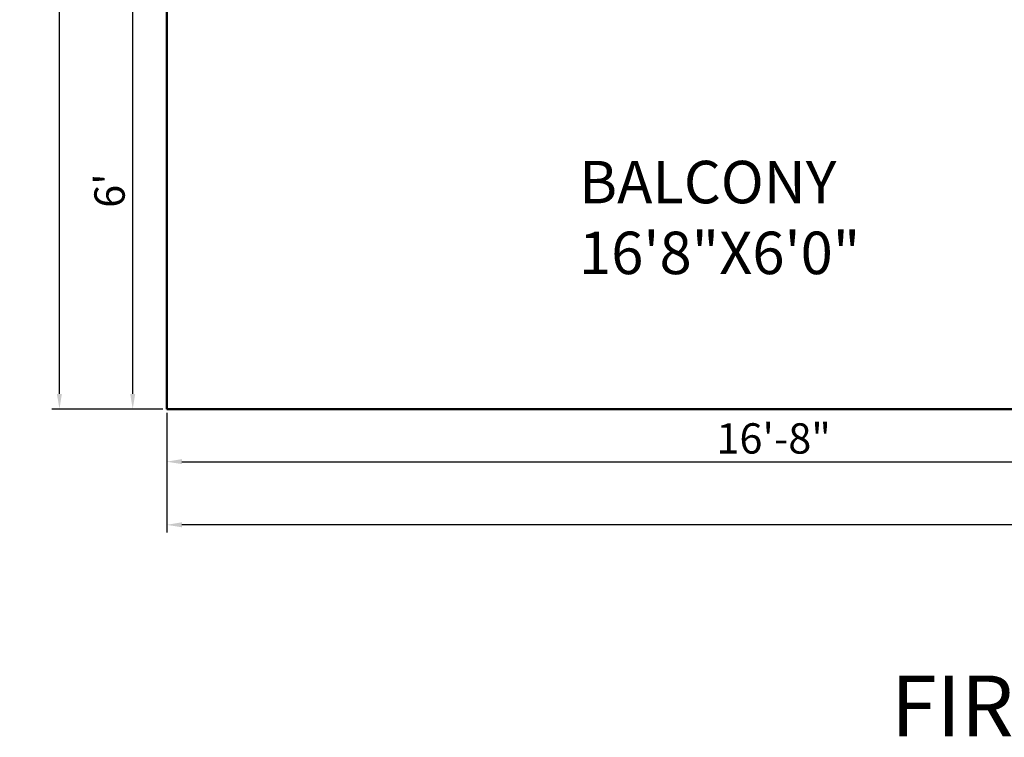
# Model space of a CAD drawing. Units: inches. Extents: x 3064 to 19385, y 846 to 15425.
# Tile 35 of 108: x 5167 to 5329, y 846 to 964. Entities that reach past the tile are written whole.
import ezdxf

# ---------------------------------------------------------------- set-up
doc = ezdxf.new("R2010")
doc.units = ezdxf.units.IN
for name, color, linetype, lineweight in [('A-ANNO-DIMS', 2, 'Continuous', 18), ('A-ANNO-TEXT', 7, 'Continuous', 25), ('A-AREA-IDEN', 3, 'Continuous', 18), ('A-WALL', 7, 'Continuous', 50)]:
    doc.layers.add(name, color=color, linetype=linetype, lineweight=lineweight)
doc.styles.get("Standard").update_dxf_attribs({"font": 'arial.ttf'})
doc.dimstyles.new('ISO-25', dxfattribs={"dimtxt": 9, "dimasz": 2.5, "dimexe": 1.25, "dimexo": 0.625, "dimtad": 1, "dimdec": 1, "dimlunit": 3, "dimtxsty": 'Standard', "dimcen": 2.5, "dimadec": 0, "dimazin": 0, "dimtfac": 1, "dimtdec": 1, "dimtmove": 0, "dimatfit": 3, "dimfxl": 1, "dimarcsym": 0})

# ---------------------------------------------------------------- blocks, each defined once
blk = doc.blocks.new('*D68')
at = {"layer": 'A-ANNO-DIMS', "color": 0, "lineweight": -2, "transparency": 16777216}
for p, q in [((5190.39, 972.1), (5184.17, 972.1)), ((5185.42, 902.6), (5185.42, 969.6)), ((5190.39, 900.1), (5184.17, 900.1))]:
    blk.add_line(p, q, dxfattribs=at)
at = {"layer": 'A-ANNO-DIMS', "color": 0, "transparency": 16777216}
for points in [[(5185, 969.6), (5185.83, 969.6), (5185.42, 972.1)], [(5185, 902.6), (5185.83, 902.6), (5185.42, 900.1)]]:
    blk.add_solid(points, dxfattribs=at)
at = {"layer": 'Defpoints', "color": 0, "transparency": 16777216}
for p in [(5185.42, 972.1), (5191.02, 972.1), (5191.02, 900.1)]:
    blk.add_point(p, dxfattribs=at)
at = {"layer": 'A-ANNO-DIMS', "color": 0, "transparency": 16777216, "insert": (5182.24, 936.1), "char_height": 5, "attachment_point": 5, "rotation": 90}
blk.add_mtext("6'", dxfattribs=at)
blk = doc.blocks.new('*D76')
at = {"layer": 'A-ANNO-DIMS', "color": 0, "lineweight": -2, "transparency": 16777216}
for p, q in [((5190.39, 1392.1), (5172.09, 1392.1)), ((5173.34, 902.6), (5173.34, 1389.6)), ((5190.39, 900.1), (5172.09, 900.1))]:
    blk.add_line(p, q, dxfattribs=at)
at = {"layer": 'A-ANNO-DIMS', "color": 0, "transparency": 16777216}
for points in [[(5172.92, 1389.6), (5173.75, 1389.6), (5173.34, 1392.1)], [(5172.92, 902.6), (5173.75, 902.6), (5173.34, 900.1)]]:
    blk.add_solid(points, dxfattribs=at)
at = {"layer": 'Defpoints', "color": 0, "transparency": 16777216}
for p in [(5173.34, 1392.1), (5191.02, 1392.1), (5191.02, 900.1)]:
    blk.add_point(p, dxfattribs=at)
at = {"layer": 'A-ANNO-DIMS', "color": 0, "transparency": 16777216, "insert": (5170.2, 1146.1), "char_height": 5, "attachment_point": 5, "rotation": 90}
blk.add_mtext("41'", dxfattribs=at)
blk = doc.blocks.new('*D77')
at = {"layer": 'A-ANNO-DIMS', "color": 0, "lineweight": -2, "transparency": 16777216}
for p, q in [((5191.02, 899.47), (5191.02, 890.17)), ((5391.02, 899.47), (5391.02, 890.17)), ((5193.52, 891.42), (5388.52, 891.42))]:
    blk.add_line(p, q, dxfattribs=at)
at = {"layer": 'A-ANNO-DIMS', "color": 0, "transparency": 16777216}
for points in [[(5193.52, 891.84), (5193.52, 891.01), (5191.02, 891.42)], [(5388.52, 891.84), (5388.52, 891.01), (5391.02, 891.42)]]:
    blk.add_solid(points, dxfattribs=at)
at = {"layer": 'Defpoints', "color": 0, "transparency": 16777216}
for p in [(5191.02, 900.1), (5391.02, 900.1), (5391.02, 891.42)]:
    blk.add_point(p, dxfattribs=at)
at = {"layer": 'A-ANNO-DIMS', "color": 0, "transparency": 16777216, "insert": (5291.02, 894.6), "char_height": 5, "attachment_point": 5}
blk.add_mtext('16\'-8"', dxfattribs=at)
blk = doc.blocks.new('*D79')
at = {"layer": 'A-ANNO-DIMS', "color": 0, "lineweight": -2, "transparency": 16777216}
for p, q in [((5191.02, 899.47), (5191.02, 879.76)), ((5533.02, 899.47), (5533.02, 879.76)), ((5530.52, 881.01), (5193.52, 881.01))]:
    blk.add_line(p, q, dxfattribs=at)
at = {"layer": 'A-ANNO-DIMS', "color": 0, "transparency": 16777216}
for points in [[(5193.52, 881.43), (5193.52, 880.6), (5191.02, 881.01)], [(5530.52, 881.43), (5530.52, 880.6), (5533.02, 881.01)]]:
    blk.add_solid(points, dxfattribs=at)
at = {"layer": 'Defpoints', "color": 0, "transparency": 16777216}
for p in [(5191.02, 900.1), (5533.02, 900.1), (5191.02, 881.01)]:
    blk.add_point(p, dxfattribs=at)
at = {"layer": 'A-ANNO-DIMS', "color": 0, "transparency": 16777216, "insert": (5362.02, 884.19), "char_height": 5, "attachment_point": 5}
blk.add_mtext('28\'-6"', dxfattribs=at)

msp = doc.modelspace()

# ---------------------------------------------------------------- linework, layer by layer
at = {"layer": 'A-WALL'}
for p, q in [((5191.02, 972.1), (5191.02, 900.1)), ((5191.02, 900.1), (5533.02, 900.1))]:
    msp.add_line(p, q, dxfattribs=at)

# ---------------------------------------------------------------- texts
at = {"layer": 'A-ANNO-TEXT', "insert": (5310.36, 856.17), "char_height": 10, "attachment_point": 1}
msp.add_mtext_dynamic_manual_height_columns('FIRST FLOOR PLAN', width=200.9739, gutter_width=12.5, heights=[0], dxfattribs=at)
at = {"layer": 'A-AREA-IDEN', "insert": (5258.95, 941), "char_height": 7, "attachment_point": 1}
msp.add_mtext_dynamic_manual_height_columns('BALCONY\\P16\'8"X6\'0"', width=67.5924, gutter_width=12.5, heights=[0], dxfattribs=at)

# ---------------------------------------------------------------- dimensions: what is measured, and where the dimension line sits
at = {"layer": 'A-ANNO-DIMS'}
for base, p2, picture, middle in [((5173.34, 1392.1), (5191.02, 1392.1), '*D76', (5170.2, 1146.1)), ((5185.42, 972.1), (5191.02, 972.1), '*D68', (5182.24, 936.1))]:
    dim = msp.add_linear_dim(base=base, p1=(5191.02, 900.1), p2=p2, angle=90, dimstyle='ISO-25', override={"dimtxt": 5, "dimclrd": 0, "dimclre": 0, "dimclrt": 0}, dxfattribs=at)
    dim.commit()
    dim.dimension.update_dxf_attribs({"geometry": picture, "text_midpoint": middle})
for base, p1, p2, picture, middle in [((5391.02, 891.42), (5191.02, 900.1), (5391.02, 900.1), '*D77', (5291.02, 894.6)), ((5191.02, 881.01), (5533.02, 900.1), (5191.02, 900.1), '*D79', (5362.02, 884.19))]:
    dim = msp.add_linear_dim(base=base, p1=p1, p2=p2, dimstyle='ISO-25', override={"dimtxt": 5, "dimclrd": 0, "dimclre": 0, "dimclrt": 0}, dxfattribs=at)
    dim.commit()
    dim.dimension.update_dxf_attribs({"geometry": picture, "text_midpoint": middle})

doc.saveas('drawing.dxf')
